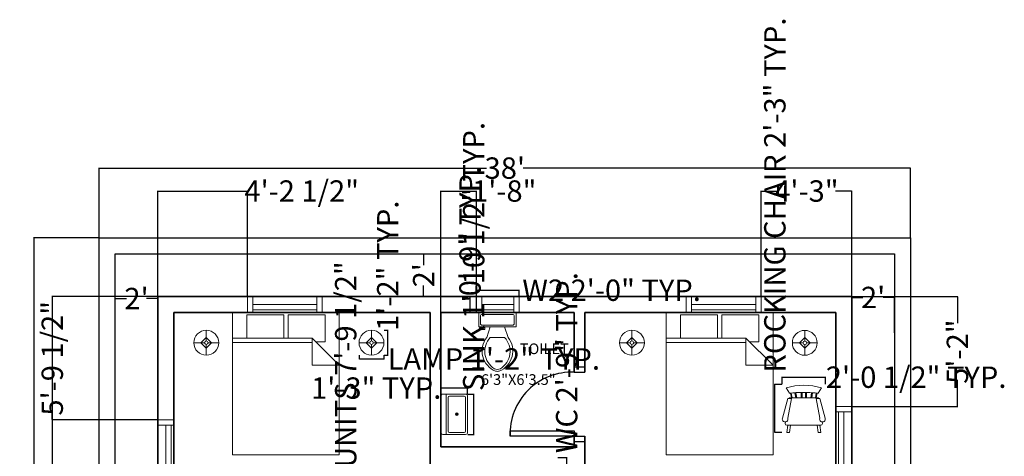
# Model space of a CAD drawing. Units: inches. Extents: x -107 to 531, y -526 to 131.
# Tile 4 of 4: x -23 to 531, y -114 to 131. Entities that reach past the tile are written whole.
import ezdxf

# ---------------------------------------------------------------- set-up
doc = ezdxf.new("R2010")
doc.units = ezdxf.units.IN
doc.header["$MEASUREMENT"] = 0
for name, color, linetype, lineweight in [('A-ANNO-DIMS', 2, 'Continuous', 18), ('A-AREA-IDEN', 7, 'Continuous', 25), ('A-DOOR', 3, 'Continuous', 25), ('A-FLOR-FIXT', 9, 'Continuous', 18), ('A-FURN', 8, 'Continuous', 18), ('A-GLAZ', 4, 'Continuous', 18), ('A-WALL', 7, 'Continuous', 35), ('C-PROP', 8, 'Continuous', 25)]:
    doc.layers.add(name, color=color, linetype=linetype, lineweight=lineweight)
doc.styles.get("Standard").update_dxf_attribs({"font": 'arial.ttf'})
doc.dimstyles.get("Standard").update_dxf_attribs({"dimtxt": 12, "dimasz": 0.18, "dimexe": 0.18, "dimexo": 0.0625, "dimgap": 0.09, "dimtad": 0, "dimdec": 1, "dimzin": 0, "dimdsep": 46, "dimlunit": 3, "dimtxsty": 'Standard', "dimcen": 0.09, "dimadec": 0, "dimazin": 0, "dimtfac": 1, "dimtdec": 1, "dimtofl": 0, "dimtmove": 0, "dimatfit": 3, "dimfxl": 1, "dimtolj": 1, "dimtzin": 0, "dimarcsym": 0})

# ---------------------------------------------------------------- blocks, each defined once
blk = doc.blocks.new('*D1')
at = {"layer": 'A-ANNO-DIMS', "color": 0, "lineweight": -2, "transparency": 16777216}
for p, q in [((21.95, 8.7), (21.95, 48.06)), ((22.13, 47.88), (239.68, 47.88)), ((477.77, 47.88), (260.22, 47.88)), ((477.95, 8.7), (477.95, 48.06))]:
    blk.add_line(p, q, dxfattribs=at)
at = {"layer": 'A-ANNO-DIMS', "color": 0, "transparency": 16777216}
for points in [[(22.13, 47.91), (22.13, 47.85), (21.95, 47.88)], [(477.77, 47.91), (477.77, 47.85), (477.95, 47.88)]]:
    blk.add_solid(points, dxfattribs=at)
at = {"layer": 'Defpoints', "color": 0, "transparency": 16777216}
for p in [(477.95, 47.88), (21.95, 8.64), (477.95, 8.64)]:
    blk.add_point(p, dxfattribs=at)
at = {"layer": 'A-ANNO-DIMS', "color": 0, "transparency": 16777216, "insert": (249.95, 47.88), "char_height": 12, "attachment_point": 5}
blk.add_mtext("\\A1;38'", dxfattribs=at)
blk = doc.blocks.new('Bed - Queen')
for p, q in [((0, -80.00003), (0, 0)), ((0, 0), (59.99999, 0)), ((59.99999, 0), (59.99999, -80.00003)), ((7.99999, -1.2), (28.79998, -1.2)), ((7.99999, -14.4), (7.99999, -1.2)), ((28.79998, -1.2), (28.79998, -14.4)), ((31.19999, -1.2), (51.99999, -1.2)), ((31.19999, -14.4), (31.19999, -1.2)), ((51.99999, -1.2), (51.99999, -16.4)), ((0, -14.4), (44.8, -14.4)), ((59.99999, -29.6), (44.8, -14.4)), ((44.8, -14.4), (44.8, -29.6)), ((51.99999, -16.4), (46.79936, -16.4)), ((44.8, -16.8), (0, -16.8)), ((44.8, -29.6), (59.99999, -29.6)), ((59.99999, -80.00003), (0, -80.00003))]:
    blk.add_line(p, q)
blk = doc.blocks.new('Lamp - Table')
for p, q in [((0, 7), (0, 1)), ((-1, 0), (-7, 0)), ((0, 3), (-3, 0)), ((-3, 0), (0, -3)), ((3, 0), (0, 3)), ((0, -3), (3, 0)), ((1, 0), (7, 0)), ((0, -1), (0, -7))]:
    blk.add_line(p, q)
for radius in [7, 1]:
    blk.add_circle((0, 0), radius)
blk = doc.blocks.new('Toilet - top')
for p, q in [((9.5, -6), (9.5, -2)), ((-10, -8.5), (-8, -8.5)), ((-10, -9.5), (-10, -8.5)), ((-7, -9.5), (-10, -9.5)), ((-8, -8.5), (-8, -8)), ((-7, -8), (-7, -9.5)), ((-4, -8), (-6, -14)), ((4, -8), (6, -14)), ((4, -14), (-4, -14))]:
    blk.add_line(p, q)
blk.add_lwpolyline([(10.5, -8), (10.5, 0), (-10.5, 0), (-10.5, -8)], close=True)
for points in [[(-9.5, -2), (-9.5, -6)], [(8.5, -1), (-8.5, -1)], [(-8.5, -7), (8.5, -7)]]:
    blk.add_lwpolyline(points)
for centre, radius, start, end in [((-8.62, -1.88), 0.884, 81.8699, 188.1301), ((8.62, -1.88), 0.884, 351.8699, 98.1301), ((-8.62, -6.12), 0.884, 171.8699, 278.1301), ((8.62, -6.12), 0.884, 261.8699, 8.1301), ((3.52, -21.58), 12.17, 141.4691, 247.9714), ((4.2, -21.82), 11.33, 136.3677, 238.9468), ((-3.52, -21.58), 12.17, 292.0284, 38.5307), ((-4.2, -21.82), 11.33, 301.053, 43.6321), ((0, -27.88), 4, 245.7318, 294.2682), ((0, -29), 4, 254.8605, 285.1395)]:
    blk.add_arc(centre, radius, start, end)
blk = doc.blocks.new('Sink-single - 30 in top')
blk.add_line((-15, -3.999996), (15, -3.999996))
for points in [[(-13.5, 0), (13.5, 0)], [(-15, -18.499996), (-15, -1.5)], [(-13.5, -17.499996), (-13.5, -6.499996)], [(-12.5, -5.499996), (12.5, -5.499996)], [(13.5, -6.499996), (13.5, -17.499996)], [(15, -1.5), (15, -18.499996)], [(13.5, -19.999996), (-13.5, -19.999996)], [(12.5, -18.499996), (-12.5, -18.499996)]]:
    blk.add_lwpolyline(points)
for radius in [1, 0.5]:
    blk.add_circle((0, -11.999996), radius)
for centre, radius, start, end in [((-13.5, -1.5), 1.5, 90, 180), ((-12.5, -6.499996), 1, 90, 180), ((12.5, -6.499996), 1, 0, 90), ((13.5, -1.5), 1.5, 0, 90), ((-13.5, -18.499996), 1.5, 180, 270), ((-12.5, -17.499996), 1, 180, 270), ((12.5, -17.499996), 1, 270, 0), ((13.5, -18.499996), 1.5, 270, 0)]:
    blk.add_arc(centre, radius, start, end)
blk = doc.blocks.new('*D13')
at = {"layer": 'A-ANNO-DIMS', "color": 0, "lineweight": -2, "transparency": 16777216}
for p, q in [((444.95, -44.8), (444.95, -24.66)), ((445.13, -24.84), (451.24, -24.84)), ((468.77, -24.84), (462.66, -24.84)), ((468.95, -44.8), (468.95, -24.66))]:
    blk.add_line(p, q, dxfattribs=at)
at = {"layer": 'A-ANNO-DIMS', "color": 0, "transparency": 16777216}
for points in [[(445.13, -24.81), (445.13, -24.87), (444.95, -24.84)], [(468.77, -24.81), (468.77, -24.87), (468.95, -24.84)]]:
    blk.add_solid(points, dxfattribs=at)
at = {"layer": 'Defpoints', "color": 0, "transparency": 16777216}
for p in [(468.95, -24.84), (444.95, -44.86), (468.95, -44.86)]:
    blk.add_point(p, dxfattribs=at)
at = {"layer": 'A-ANNO-DIMS', "color": 0, "transparency": 16777216, "insert": (456.95, -24.84), "char_height": 12, "attachment_point": 5}
blk.add_mtext("\\A1;2'", dxfattribs=at)
blk = doc.blocks.new('*D14')
at = {"layer": 'A-ANNO-DIMS', "color": 0, "lineweight": -2, "transparency": 16777216}
for p, q in [((30.95, -34.2), (30.95, -25.25)), ((31.13, -25.43), (37.24, -25.43)), ((54.77, -25.43), (48.66, -25.43)), ((54.95, -34.2), (54.95, -25.25))]:
    blk.add_line(p, q, dxfattribs=at)
at = {"layer": 'A-ANNO-DIMS', "color": 0, "transparency": 16777216}
for points in [[(31.13, -25.4), (31.13, -25.46), (30.95, -25.43)], [(54.77, -25.4), (54.77, -25.46), (54.95, -25.43)]]:
    blk.add_solid(points, dxfattribs=at)
at = {"layer": 'Defpoints', "color": 0, "transparency": 16777216}
for p in [(30.95, -25.43), (30.95, -34.26), (54.95, -34.26)]:
    blk.add_point(p, dxfattribs=at)
at = {"layer": 'A-ANNO-DIMS', "color": 0, "transparency": 16777216, "insert": (42.95, -25.43), "char_height": 12, "attachment_point": 5}
blk.add_mtext("\\A1;2'", dxfattribs=at)
blk = doc.blocks.new('*D15')
at = {"layer": 'A-ANNO-DIMS', "color": 0, "lineweight": -2, "transparency": 16777216}
for p, q in [((196.15, -0.36), (204.52, -0.36)), ((204.34, -0.54), (204.34, -6.65)), ((204.34, -24.18), (204.34, -18.08)), ((196.15, -24.36), (204.52, -24.36))]:
    blk.add_line(p, q, dxfattribs=at)
at = {"layer": 'A-ANNO-DIMS', "color": 0, "transparency": 16777216}
for points in [[(204.31, -0.54), (204.37, -0.54), (204.34, -0.36)], [(204.31, -24.18), (204.37, -24.18), (204.34, -24.36)]]:
    blk.add_solid(points, dxfattribs=at)
at = {"layer": 'Defpoints', "color": 0, "transparency": 16777216}
for p in [(196.09, -0.36), (204.34, -0.36), (196.09, -24.36)]:
    blk.add_point(p, dxfattribs=at)
at = {"layer": 'A-ANNO-DIMS', "color": 0, "transparency": 16777216, "insert": (204.34, -12.36), "char_height": 12, "attachment_point": 5, "rotation": 90}
blk.add_mtext("\\A1;2'", dxfattribs=at)
blk = doc.blocks.new('Chair - Rocking')
for p, q in [((-8, -4.5), (-10, -1.5)), ((-7.5, -4.5), (-7, -7)), ((-6.5, -7), (-7.02225, -4.43)), ((-4.5, -7), (-4.96674, -4.19951)), ((-4, -7), (-4.40532, -4.16272)), ((-1.5, -4.05012), (-1.5, -7)), ((-1, -7), (-1, -4.05012)), ((1, -7), (1, -4.04655)), ((1.5, -4.05012), (1.5, -7)), ((4, -7), (4.40187, -4.18694)), ((4.5, -7), (4.96761, -4.19437)), ((6.5, -7), (7, -4.4057)), ((7.5, -4.5), (7, -7)), ((8, -4.5), (10, -1.5)), ((-9, -7.5), (-12, -18.49999)), ((-7, -7.5), (-9, -7.5)), ((-9, -18.49999), (-7, -7.5)), ((-8.23428, -6.99939), (-8.3093, -7.47958)), ((-8.23041, -7), (8.23915, -7)), ((7, -7.5), (9, -7.5)), ((9, -18.49999), (7, -7.5)), ((8.31071, -7.48854), (8.23449, -7.00073)), ((9, -7.5), (12, -18.49999)), ((-10.36644, -20.64523), (-10.5, -21.49999)), ((10.5, -21.49999), (10.3575, -20.58798)), ((-9, -22.49999), (-9.5, -26.49999)), ((0, -22.49999), (-9.5, -22.49999)), ((-9.5, -26.49999), (-8, -26.49999)), ((-8, -26.49999), (-7.5, -22.49999)), ((0, -22.49999), (9.5, -22.49999)), ((8, -26.49999), (7.5, -22.49999)), ((9.5, -26.49999), (8, -26.49999)), ((9, -22.49999), (9.5, -26.49999))]:
    blk.add_line(p, q)
for centre, radius, start, end in [((0, -34.08333), 34.08333, 72.93847, 107.0615), ((0, -68.25004), 64.25, 93.92211, 97.15267), ((0, -68.25004), 64.25, 82.84733, 93.92211), ((-10.5, -18.99999), 1.58114, 161.5651, 18.43495), ((-9.5, -21.49999), 1, 180, 270), ((10.5, -18.99999), 1.58114, 161.5651, 18.43495), ((9.5, -21.49999), 1, 270, 0)]:
    blk.add_arc(centre, radius, start, end)
blk = doc.blocks.new('*D18')
at = {"layer": 'A-ANNO-DIMS', "color": 0, "lineweight": -2, "transparency": 16777216}
for p, q in [((21.89, 8.64), (-15.01, 8.64)), ((-14.83, 8.46), (-14.83, -220.85)), ((-14.83, -471.18), (-14.83, -241.88)), ((21.89, -471.36), (-15.01, -471.36))]:
    blk.add_line(p, q, dxfattribs=at)
at = {"layer": 'A-ANNO-DIMS', "color": 0, "transparency": 16777216}
for points in [[(-14.86, 8.46), (-14.8, 8.46), (-14.83, 8.64)], [(-14.86, -471.18), (-14.8, -471.18), (-14.83, -471.36)]]:
    blk.add_solid(points, dxfattribs=at)
at = {"layer": 'Defpoints', "color": 0, "transparency": 16777216}
for p in [(21.95, 8.64), (-14.83, -471.36), (21.95, -471.36)]:
    blk.add_point(p, dxfattribs=at)
at = {"layer": 'A-ANNO-DIMS', "color": 0, "transparency": 16777216, "insert": (-14.83, -231.36), "char_height": 12, "attachment_point": 5, "rotation": 90}
blk.add_mtext("\\A1;40'", dxfattribs=at)
blk = doc.blocks.new('WIN-36')
for p, q in [((0, 0), (0, 9)), ((3, 0), (3, 9)), ((3, 9), (39, 9)), ((39, 7.5), (3, 7.5)), ((39, 9), (39, 0)), ((42, 9), (42, 0)), ((39, 4.5), (3, 4.5)), ((39, 0), (3, 0))]:
    blk.add_line(p, q)
blk = doc.blocks.new('WIN-18')
for p, q in [((0, 9), (0, 0)), ((21, 9), (3, 9)), ((3, 9), (3, 0)), ((21, 0), (21, 9)), ((24, 0), (24, 9)), ((3, 4.5), (21, 4.5)), ((3, 1.5), (21, 1.5)), ((3, 0), (21, 0))]:
    blk.add_line(p, q)
blk = doc.blocks.new('DOOR-36-SWING')
for p, q in [((36.03, 42), (42.03, 42)), ((36.03, 39), (42.03, 39)), ((36.03, 3), (42.03, 3)), ((36.03, 0), (42.03, 0))]:
    blk.add_line(p, q)
blk.add_lwpolyline([(36.03, 3), (0.03, 3), (0.03, 6), (36.03, 6)], close=True)
blk.add_arc((34.53, 4.5), 34.53, 87.5104, 182.4896)
blk = doc.blocks.new('*D25')
at = {"layer": 'A-ANNO-DIMS', "color": 0, "lineweight": -2, "transparency": 16777216}
for p, q in [((233.99, -24.3), (233.99, -20.58)), ((234.17, -20.76), (257.81, -20.76)), ((257.99, -24.3), (257.99, -20.58)), ((257.99, -20.76), (258.17, -20.76))]:
    blk.add_line(p, q, dxfattribs=at)
at = {"layer": 'A-ANNO-DIMS', "color": 0, "transparency": 16777216}
for points in [[(234.17, -20.73), (234.17, -20.79), (233.99, -20.76)], [(257.81, -20.73), (257.81, -20.79), (257.99, -20.76)]]:
    blk.add_solid(points, dxfattribs=at)
at = {"layer": 'Defpoints', "color": 0, "transparency": 16777216}
for p in [(257.99, -20.76), (233.99, -24.36), (257.99, -24.36)]:
    blk.add_point(p, dxfattribs=at)
at = {"layer": 'A-ANNO-DIMS', "color": 0, "transparency": 16777216, "insert": (309.98, -20.76), "char_height": 12, "attachment_point": 5}
blk.add_mtext('\\A1;W2 2\'-0" TYP.', dxfattribs=at)
blk = doc.blocks.new('*D26')
at = {"layer": 'A-ANNO-DIMS', "color": 0, "lineweight": -2, "transparency": 16777216}
for p, q in [((233.93, -24.36), (230.21, -24.36)), ((230.39, -24.36), (230.39, -24.18)), ((230.39, -33.18), (230.39, -24.54)), ((233.93, -33.36), (230.21, -33.36))]:
    blk.add_line(p, q, dxfattribs=at)
at = {"layer": 'A-ANNO-DIMS', "color": 0, "transparency": 16777216}
for points in [[(230.36, -24.54), (230.42, -24.54), (230.39, -24.36)], [(230.36, -33.18), (230.42, -33.18), (230.39, -33.36)]]:
    blk.add_solid(points, dxfattribs=at)
at = {"layer": 'Defpoints', "color": 0, "transparency": 16777216}
for p in [(230.39, -24.36), (233.99, -24.36), (233.99, -33.36)]:
    blk.add_point(p, dxfattribs=at)
at = {"layer": 'A-ANNO-DIMS', "color": 0, "transparency": 16777216, "insert": (230.39, 12.48), "char_height": 12, "attachment_point": 5, "rotation": 90}
blk.add_mtext('\\A1;0\'-9" TYP.', dxfattribs=at)
blk = doc.blocks.new('*D33')
at = {"layer": 'A-ANNO-DIMS', "color": 0, "lineweight": -2, "transparency": 16777216}
for p, q in [((168.03, -57.34), (168.03, -59.56)), ((168.21, -59.38), (181.85, -59.38)), ((182.03, -57.34), (182.03, -59.56)), ((182.03, -59.38), (182.21, -59.38))]:
    blk.add_line(p, q, dxfattribs=at)
at = {"layer": 'A-ANNO-DIMS', "color": 0, "transparency": 16777216}
for points in [[(168.21, -59.35), (168.21, -59.41), (168.03, -59.38)], [(181.85, -59.35), (181.85, -59.41), (182.03, -59.38)]]:
    blk.add_solid(points, dxfattribs=at)
at = {"layer": 'Defpoints', "color": 0, "transparency": 16777216}
for p in [(168.03, -57.28), (182.03, -57.28), (182.03, -59.38)]:
    blk.add_point(p, dxfattribs=at)
at = {"layer": 'A-ANNO-DIMS', "color": 0, "transparency": 16777216, "insert": (243.76, -59.38), "char_height": 12, "attachment_point": 5}
blk.add_mtext('\\A1;LAMP 1\'-2" TYP.', dxfattribs=at)
blk = doc.blocks.new('*D34')
at = {"layer": 'A-ANNO-DIMS', "color": 0, "lineweight": -2, "transparency": 16777216}
for p, q in [((182.09, -43.28), (184.31, -43.28)), ((184.13, -43.28), (184.13, -43.1)), ((184.13, -57.1), (184.13, -43.46)), ((182.09, -57.28), (184.31, -57.28))]:
    blk.add_line(p, q, dxfattribs=at)
at = {"layer": 'A-ANNO-DIMS', "color": 0, "transparency": 16777216}
for points in [[(184.1, -43.46), (184.16, -43.46), (184.13, -43.28)], [(184.1, -57.1), (184.16, -57.1), (184.13, -57.28)]]:
    blk.add_solid(points, dxfattribs=at)
at = {"layer": 'Defpoints', "color": 0, "transparency": 16777216}
for p in [(182.03, -43.28), (184.13, -43.28), (182.03, -57.28)]:
    blk.add_point(p, dxfattribs=at)
at = {"layer": 'A-ANNO-DIMS', "color": 0, "transparency": 16777216, "insert": (184.13, -7), "char_height": 12, "attachment_point": 5, "rotation": 90}
blk.add_mtext('\\A1;1\'-2" TYP.', dxfattribs=at)
blk = doc.blocks.new('*D35')
at = {"layer": 'A-ANNO-DIMS', "color": 0, "lineweight": -2, "transparency": 16777216}
for p, q in [((405.71, -73.69), (401.54, -73.69)), ((401.72, -73.69), (401.72, -73.51)), ((401.72, -100.51), (401.72, -73.87)), ((405.71, -100.69), (401.54, -100.69))]:
    blk.add_line(p, q, dxfattribs=at)
at = {"layer": 'A-ANNO-DIMS', "color": 0, "transparency": 16777216}
for points in [[(401.69, -73.87), (401.75, -73.87), (401.72, -73.69)], [(401.69, -100.51), (401.75, -100.51), (401.72, -100.69)]]:
    blk.add_solid(points, dxfattribs=at)
at = {"layer": 'Defpoints', "color": 0, "transparency": 16777216}
for p in [(401.72, -73.69), (405.77, -73.69), (405.77, -100.69)]:
    blk.add_point(p, dxfattribs=at)
at = {"layer": 'A-ANNO-DIMS', "color": 0, "transparency": 16777216, "insert": (401.72, 32.7), "char_height": 12, "attachment_point": 5, "rotation": 90}
blk.add_mtext('\\A1;ROCKING CHAIR 2\'-3" TYP.', dxfattribs=at)
blk = doc.blocks.new('*D36')
at = {"layer": 'A-ANNO-DIMS', "color": 0, "lineweight": -2, "transparency": 16777216}
for p, q in [((405.77, -73.63), (405.77, -69.46)), ((405.95, -69.64), (430.02, -69.64)), ((430.2, -73.63), (430.2, -69.46)), ((430.2, -69.64), (430.38, -69.64))]:
    blk.add_line(p, q, dxfattribs=at)
at = {"layer": 'A-ANNO-DIMS', "color": 0, "transparency": 16777216}
for points in [[(405.95, -69.61), (405.95, -69.67), (405.77, -69.64)], [(430.02, -69.61), (430.02, -69.67), (430.2, -69.64)]]:
    blk.add_solid(points, dxfattribs=at)
at = {"layer": 'Defpoints', "color": 0, "transparency": 16777216}
for p in [(430.2, -69.64), (405.77, -73.69), (430.2, -73.69)]:
    blk.add_point(p, dxfattribs=at)
at = {"layer": 'A-ANNO-DIMS', "color": 0, "transparency": 16777216, "insert": (481.13, -69.64), "char_height": 12, "attachment_point": 5}
blk.add_mtext('\\A1;2\'-0 1/2" TYP.', dxfattribs=at)
blk = doc.blocks.new('*D39')
at = {"layer": 'A-ANNO-DIMS', "color": 0, "lineweight": -2, "transparency": 16777216}
for p, q in [((229.12, -79.16), (232.64, -79.16)), ((232.46, -79.16), (232.46, -78.98)), ((232.46, -101.64), (232.46, -79.34)), ((229.12, -101.82), (232.64, -101.82))]:
    blk.add_line(p, q, dxfattribs=at)
at = {"layer": 'A-ANNO-DIMS', "color": 0, "transparency": 16777216}
for points in [[(232.43, -79.34), (232.49, -79.34), (232.46, -79.16)], [(232.43, -101.64), (232.49, -101.64), (232.46, -101.82)]]:
    blk.add_solid(points, dxfattribs=at)
at = {"layer": 'Defpoints', "color": 0, "transparency": 16777216}
for p in [(229.06, -79.16), (232.46, -79.16), (229.06, -101.82)]:
    blk.add_point(p, dxfattribs=at)
at = {"layer": 'A-ANNO-DIMS', "color": 0, "transparency": 16777216, "insert": (232.46, -1.81), "char_height": 12, "attachment_point": 5, "rotation": 90}
blk.add_mtext('\\A1;SINK 1\'-10 1/2" TYP.', dxfattribs=at)
blk = doc.blocks.new('*D40')
at = {"layer": 'A-ANNO-DIMS', "color": 0, "lineweight": -2, "transparency": 16777216}
for p, q in [((213.95, -75.76), (213.77, -75.76)), ((213.95, -79.09), (213.95, -75.58)), ((228.88, -75.76), (214.13, -75.76)), ((229.06, -79.09), (229.06, -75.58))]:
    blk.add_line(p, q, dxfattribs=at)
at = {"layer": 'A-ANNO-DIMS', "color": 0, "transparency": 16777216}
for points in [[(214.13, -75.73), (214.13, -75.79), (213.95, -75.76)], [(228.88, -75.73), (228.88, -75.79), (229.06, -75.76)]]:
    blk.add_solid(points, dxfattribs=at)
at = {"layer": 'Defpoints', "color": 0, "transparency": 16777216}
for p in [(213.95, -75.76), (213.95, -79.16), (229.06, -79.16)]:
    blk.add_point(p, dxfattribs=at)
at = {"layer": 'A-ANNO-DIMS', "color": 0, "transparency": 16777216, "insert": (177.67, -75.76), "char_height": 12, "attachment_point": 5}
blk.add_mtext('\\A1;1\'-3" TYP.', dxfattribs=at)
blk = doc.blocks.new('*D43')
at = {"layer": 'A-ANNO-DIMS', "color": 0, "lineweight": -2, "transparency": 16777216}
for p, q in [((279.83, -114.86), (284.9, -114.86)), ((284.72, -114.86), (284.72, -114.68)), ((284.72, -147.73), (284.72, -115.04)), ((279.83, -147.91), (284.9, -147.91))]:
    blk.add_line(p, q, dxfattribs=at)
at = {"layer": 'A-ANNO-DIMS', "color": 0, "transparency": 16777216}
for points in [[(284.69, -115.04), (284.75, -115.04), (284.72, -114.86)], [(284.69, -147.73), (284.75, -147.73), (284.72, -147.91)]]:
    blk.add_solid(points, dxfattribs=at)
at = {"layer": 'Defpoints', "color": 0, "transparency": 16777216}
for p in [(279.77, -114.86), (284.72, -114.86), (279.77, -147.91)]:
    blk.add_point(p, dxfattribs=at)
at = {"layer": 'A-ANNO-DIMS', "color": 0, "transparency": 16777216, "insert": (284.72, -61.48), "char_height": 12, "attachment_point": 5, "rotation": 90}
blk.add_mtext('\\A1;WC 2\'-9" TYP.', dxfattribs=at)
blk = doc.blocks.new('*D51')
at = {"layer": 'A-ANNO-DIMS', "color": 0, "lineweight": -2, "transparency": 16777216}
for p, q in [((146.59, -195.42), (160.7, -195.42)), ((160.52, -195.42), (160.52, -195.24)), ((160.52, -288.52), (160.52, -195.6)), ((146.59, -288.7), (160.7, -288.7))]:
    blk.add_line(p, q, dxfattribs=at)
at = {"layer": 'A-ANNO-DIMS', "color": 0, "transparency": 16777216}
for points in [[(160.49, -195.6), (160.55, -195.6), (160.52, -195.42)], [(160.49, -288.52), (160.55, -288.52), (160.52, -288.7)]]:
    blk.add_solid(points, dxfattribs=at)
at = {"layer": 'Defpoints', "color": 0, "transparency": 16777216}
for p in [(146.53, -195.42), (160.52, -195.42), (146.53, -288.7)]:
    blk.add_point(p, dxfattribs=at)
at = {"layer": 'A-ANNO-DIMS', "color": 0, "transparency": 16777216, "insert": (160.52, -98.9), "char_height": 12, "attachment_point": 5, "rotation": 90}
blk.add_mtext('\\A1;KITCHEN UNITS 7\'-9 1/2"', dxfattribs=at)
blk = doc.blocks.new('*D60')
at = {"layer": 'A-ANNO-DIMS', "color": 0, "lineweight": -2, "transparency": 16777216}
for p, q in [((54.89, -24.36), (-4.58, -24.36)), ((-4.4, -24.54), (-4.4, -227.16)), ((-4.4, -471.18), (-4.4, -268.56)), ((21.89, -471.36), (-4.58, -471.36))]:
    blk.add_line(p, q, dxfattribs=at)
at = {"layer": 'A-ANNO-DIMS', "color": 0, "transparency": 16777216}
for points in [[(-4.43, -24.54), (-4.37, -24.54), (-4.4, -24.36)], [(-4.43, -471.18), (-4.37, -471.18), (-4.4, -471.36)]]:
    blk.add_solid(points, dxfattribs=at)
at = {"layer": 'Defpoints', "color": 0, "transparency": 16777216}
for p in [(54.95, -24.36), (-4.4, -471.36), (21.95, -471.36)]:
    blk.add_point(p, dxfattribs=at)
at = {"layer": 'A-ANNO-DIMS', "color": 0, "transparency": 16777216, "insert": (-4.4, -247.86), "char_height": 12, "attachment_point": 5, "rotation": 90}
blk.add_mtext('\\A1;37\'-3"', dxfattribs=at)
blk = doc.blocks.new('*D63')
at = {"layer": 'A-ANNO-DIMS', "color": 0, "lineweight": -2, "transparency": 16777216}
for p, q in [((54.95, -24.3), (54.95, 35.17)), ((55.13, 34.99), (105.17, 34.99)), ((105.35, -24.3), (105.35, 35.17)), ((105.35, 34.99), (105.53, 34.99))]:
    blk.add_line(p, q, dxfattribs=at)
at = {"layer": 'A-ANNO-DIMS', "color": 0, "transparency": 16777216}
for points in [[(55.13, 35.02), (55.13, 34.96), (54.95, 34.99)], [(105.17, 35.02), (105.17, 34.96), (105.35, 34.99)]]:
    blk.add_solid(points, dxfattribs=at)
at = {"layer": 'Defpoints', "color": 0, "transparency": 16777216}
for p in [(105.35, 34.99), (54.95, -24.36), (105.35, -24.36)]:
    blk.add_point(p, dxfattribs=at)
at = {"layer": 'A-ANNO-DIMS', "color": 0, "transparency": 16777216, "insert": (135.79, 34.99), "char_height": 12, "attachment_point": 5}
blk.add_mtext('\\A1;4\'-2 1/2"', dxfattribs=at)
blk = doc.blocks.new('*D64')
at = {"layer": 'A-ANNO-DIMS', "color": 0, "lineweight": -2, "transparency": 16777216}
for p, q in [((393.96, -24.3), (393.96, 35.17)), ((394.14, 34.99), (403.17, 34.99)), ((444.77, 34.99), (435.74, 34.99)), ((444.95, -24.3), (444.95, 35.17))]:
    blk.add_line(p, q, dxfattribs=at)
at = {"layer": 'A-ANNO-DIMS', "color": 0, "transparency": 16777216}
for points in [[(394.14, 35.02), (394.14, 34.96), (393.96, 34.99)], [(444.77, 35.02), (444.77, 34.96), (444.95, 34.99)]]:
    blk.add_solid(points, dxfattribs=at)
at = {"layer": 'Defpoints', "color": 0, "transparency": 16777216}
for p in [(444.95, 34.99), (393.96, -24.36), (444.95, -24.36)]:
    blk.add_point(p, dxfattribs=at)
at = {"layer": 'A-ANNO-DIMS', "color": 0, "transparency": 16777216, "insert": (419.46, 34.99), "char_height": 12, "attachment_point": 5}
blk.add_mtext('\\A1;4\'-3"', dxfattribs=at)
blk = doc.blocks.new('*D65')
at = {"layer": 'A-ANNO-DIMS', "color": 0, "lineweight": -2, "transparency": 16777216}
for p, q in [((213.95, -33.3), (213.95, 35.17)), ((214.13, 34.99), (233.81, 34.99)), ((233.99, -33.3), (233.99, 35.17)), ((233.99, 34.99), (234.17, 34.99))]:
    blk.add_line(p, q, dxfattribs=at)
at = {"layer": 'A-ANNO-DIMS', "color": 0, "transparency": 16777216}
for points in [[(214.13, 35.02), (214.13, 34.96), (213.95, 34.99)], [(233.81, 35.02), (233.81, 34.96), (233.99, 34.99)]]:
    blk.add_solid(points, dxfattribs=at)
at = {"layer": 'Defpoints', "color": 0, "transparency": 16777216}
for p in [(233.99, 34.99), (213.95, -33.36), (233.99, -33.36)]:
    blk.add_point(p, dxfattribs=at)
at = {"layer": 'A-ANNO-DIMS', "color": 0, "transparency": 16777216, "insert": (249.64, 34.99), "char_height": 12, "attachment_point": 5}
blk.add_mtext('\\A1;1\'-8"', dxfattribs=at)
blk = doc.blocks.new('*D70')
at = {"layer": 'A-ANNO-DIMS', "color": 0, "lineweight": -2, "transparency": 16777216}
for p, q in [((54.89, -24.36), (-4.58, -24.36)), ((-4.4, -24.54), (-4.4, -29)), ((54.89, -93.68), (-4.58, -93.68)), ((-4.4, -93.5), (-4.4, -89.04))]:
    blk.add_line(p, q, dxfattribs=at)
at = {"layer": 'A-ANNO-DIMS', "color": 0, "transparency": 16777216}
for points in [[(-4.43, -24.54), (-4.37, -24.54), (-4.4, -24.36)], [(-4.43, -93.5), (-4.37, -93.5), (-4.4, -93.68)]]:
    blk.add_solid(points, dxfattribs=at)
at = {"layer": 'Defpoints', "color": 0, "transparency": 16777216}
for p in [(54.95, -24.36), (-4.4, -93.68), (54.95, -93.68)]:
    blk.add_point(p, dxfattribs=at)
at = {"layer": 'A-ANNO-DIMS', "color": 0, "transparency": 16777216, "insert": (-4.4, -59.02), "char_height": 12, "attachment_point": 5, "rotation": 90}
blk.add_mtext('\\A1;5\'-9 1/2"', dxfattribs=at)
blk = doc.blocks.new('*D73')
at = {"layer": 'A-ANNO-DIMS', "color": 0, "lineweight": -2, "transparency": 16777216}
for p, q in [((445.01, -24.36), (504.48, -24.36)), ((504.3, -24.54), (504.3, -39.23)), ((504.3, -85.99), (504.3, -71.3)), ((445.01, -86.17), (504.48, -86.17))]:
    blk.add_line(p, q, dxfattribs=at)
at = {"layer": 'A-ANNO-DIMS', "color": 0, "transparency": 16777216}
for points in [[(504.27, -24.54), (504.33, -24.54), (504.3, -24.36)], [(504.27, -85.99), (504.33, -85.99), (504.3, -86.17)]]:
    blk.add_solid(points, dxfattribs=at)
at = {"layer": 'Defpoints', "color": 0, "transparency": 16777216}
for p in [(444.95, -24.36), (444.95, -86.17), (504.3, -86.17)]:
    blk.add_point(p, dxfattribs=at)
at = {"layer": 'A-ANNO-DIMS', "color": 0, "transparency": 16777216, "insert": (504.3, -55.27), "char_height": 12, "attachment_point": 5, "rotation": 90}
blk.add_mtext('\\A1;5\'-2"', dxfattribs=at)

msp = doc.modelspace()

# ---------------------------------------------------------------- linework, layer by layer
at = {"layer": 'A-WALL'}
for p, q in [((54.95, -462.36), (54.95, -24.36)), ((54.95, -24.36), (444.95, -24.36)), ((444.95, -24.36), (444.95, -462.36)), ((63.95, -33.36), (207.95, -33.36)), ((63.95, -189.36), (63.95, -33.36)), ((207.95, -120.86), (207.95, -33.36)), ((213.95, -108.86), (213.95, -33.36)), ((213.95, -33.36), (288.95, -33.36)), ((288.95, -66.86), (288.95, -33.36)), ((294.95, -66.86), (294.95, -33.36)), ((294.95, -33.36), (435.95, -33.36)), ((435.95, -33.36), (435.95, -189.36)), ((288.95, -108.86), (288.95, -102.86)), ((294.95, -189.36), (294.95, -102.86)), ((213.95, -108.86), (288.95, -108.86))]:
    msp.add_line(p, q, dxfattribs=at)
at = {"layer": 'C-PROP'}
for p, q in [((30.95, -0.36), (468.95, -0.36)), ((30.95, -462.36), (30.95, -0.36)), ((468.95, -0.36), (468.95, -462.36))]:
    msp.add_line(p, q, dxfattribs=at)
msp.add_lwpolyline([(231.95, -471.36), (21.95, -471.36), (21.95, 8.64), (477.95, 8.64), (477.95, -471.36), (303.95, -471.36)], dxfattribs=at)

# ---------------------------------------------------------------- block references
at = {"layer": 'A-DOOR'}
msp.add_blockref('DOOR-36-SWING', (252.92, -105.86), dxfattribs=at)
at = {"layer": 'A-FLOR-FIXT'}
msp.add_blockref('Toilet - top', (245.8, -33.36), dxfattribs=at)
at = {"layer": 'A-FLOR-FIXT', "xscale": 0.7554348055935636, "yscale": 0.7554348055935636, "zscale": 0.7554348055935636, "rotation": 90}
msp.add_blockref('Sink-single - 30 in top', (213.95, -90.49), dxfattribs=at)
at = {"layer": 'A-FURN'}
for name, p in [('Bed - Queen', (96.92, -33.36)), ('Bed - Queen', (340.7, -33.36)), ('Lamp - Table', (82.18, -50.28)), ('Lamp - Table', (175.03, -50.28)), ('Lamp - Table', (321.39, -50.28)), ('Lamp - Table', (418.55, -50.34)), ('Chair - Rocking', (417.99, -74.19))]:
    msp.add_blockref(name, p, dxfattribs=at)
at = {"layer": 'A-GLAZ'}
for p, rotation in [((147.35, -24.36), 180), ((393.96, -24.36), 180), ((444.95, -128.17), 89.99999999999987), ((54.95, -93.68), 270.0000000000002)]:
    msp.add_blockref('WIN-36', p, dxfattribs=dict(at, rotation=rotation))
msp.add_blockref('WIN-18', (233.99, -33.36), dxfattribs=at)

# ---------------------------------------------------------------- texts
at = {"layer": 'A-AREA-IDEN'}
for s, p in [('TOILET', (258.36, -56.68)), ('6\'3"X6\'3.5"', (236.54, -73.97))]:
    msp.add_text(s, height=6, dxfattribs=at).set_placement(p)

# ---------------------------------------------------------------- dimensions: what is measured, and where the dimension line sits
at = {"layer": 'A-ANNO-DIMS'}
for base, p1, p2, angle, text, picture, middle in [((401.72, -73.69), (405.77, -100.69), (405.77, -73.69), 90, 'ROCKING CHAIR <> TYP.', '*D35', (401.72, 32.7)), ((232.46, -79.16), (229.06, -101.82), (229.06, -79.16), 90, 'SINK <> TYP.', '*D39', (232.46, -1.81)), ((230.39, -24.36), (233.99, -33.36), (233.99, -24.36), 90, '<> TYP.', '*D26', (230.39, 12.48)), ((184.13, -43.28), (182.03, -57.28), (182.03, -43.28), 90, '<> TYP.', '*D34', (184.13, -7)), ((160.52, -195.42), (146.53, -288.7), (146.53, -195.42), 90, 'KITCHEN UNITS <>', '*D51', (160.52, -98.9)), ((284.7239, -114.8618), (279.7669, -147.9081), (279.7669, -114.8618), 90, 'WC <> TYP.', '*D43', (284.7239, -61.48)), ((213.95, -75.76), (229.06, -79.16), (213.95, -79.16), 180, '<> TYP.', '*D40', (177.67, -75.76))]:
    dim = msp.add_linear_dim(base=base, p1=p1, p2=p2, angle=angle, text=text, dimstyle='Standard', override={"dimdec": 1, "dimlfac": 1, "dimrnd": 0, "dimzin": 1, "dimdsep": 46, "dimlunit": 4, "dimfrac": 2}, dxfattribs=at)
    dim.commit()
    dim.dimension.update_dxf_attribs({"geometry": picture, "text_midpoint": middle})
for base, p1, p2, override, picture, middle in [((477.95, 47.88), (21.95, 8.64), (477.95, 8.64), {"dimclrd": 0, "dimclre": 0, "dimclrt": 0}, '*D1', (249.95, 47.88)), ((105.35, 34.99), (54.95, -24.36), (105.35, -24.36), {"dimdec": 1, "dimlfac": 1, "dimrnd": 0, "dimzin": 1, "dimdsep": 46, "dimlunit": 4, "dimfrac": 2}, '*D63', (135.79, 34.99)), ((233.99, 34.99), (213.95, -33.36), (233.99, -33.36), {"dimdec": 1, "dimlfac": 1, "dimrnd": 0, "dimzin": 1, "dimdsep": 46, "dimlunit": 4, "dimfrac": 2}, '*D65', (249.64, 34.99)), ((444.95, 34.99), (393.96, -24.36), (444.95, -24.36), {"dimdec": 1, "dimlfac": 1, "dimrnd": 0, "dimzin": 1, "dimdsep": 46, "dimlunit": 4, "dimfrac": 2}, '*D64', (419.46, 34.99)), ((30.95, -25.43), (54.95, -34.26), (30.95, -34.26), {"dimclrd": 0, "dimclre": 0, "dimclrt": 0}, '*D14', (42.95, -25.43)), ((468.95, -24.84), (444.95, -44.86), (468.95, -44.86), {"dimclrd": 0, "dimclre": 0, "dimclrt": 0}, '*D13', (456.95, -24.84))]:
    dim = msp.add_linear_dim(base=base, p1=p1, p2=p2, dimstyle='Standard', override=override, dxfattribs=at)
    dim.commit()
    dim.dimension.update_dxf_attribs({"geometry": picture, "text_midpoint": middle})
for base, p1, p2, override, picture, middle in [((-14.83, -471.36), (21.95, 8.64), (21.95, -471.36), {"dimclrd": 0, "dimclre": 0, "dimclrt": 0}, '*D18', (-14.83, -231.36)), ((204.34, -0.36), (196.09, -24.36), (196.09, -0.36), {"dimclrd": 0, "dimclre": 0, "dimclrt": 0}, '*D15', (204.34, -12.36)), ((-4.4, -93.68), (54.95, -24.36), (54.95, -93.68), {"dimdec": 1, "dimlfac": 1, "dimrnd": 0, "dimzin": 1, "dimdsep": 46, "dimlunit": 4, "dimfrac": 2}, '*D70', (-4.4, -59.02)), ((-4.4, -471.36), (54.95, -24.36), (21.95, -471.36), {"dimdec": 1, "dimlfac": 1, "dimrnd": 0, "dimzin": 1, "dimdsep": 46, "dimlunit": 4, "dimfrac": 2}, '*D60', (-4.4, -247.86)), ((504.3, -86.17), (444.95, -24.36), (444.95, -86.17), {"dimdec": 1, "dimlfac": 1, "dimrnd": 0, "dimzin": 1, "dimdsep": 46, "dimlunit": 4, "dimfrac": 2}, '*D73', (504.3, -55.27))]:
    dim = msp.add_linear_dim(base=base, p1=p1, p2=p2, angle=90, dimstyle='Standard', override=override, dxfattribs=at)
    dim.commit()
    dim.dimension.update_dxf_attribs({"geometry": picture, "text_midpoint": middle})
for base, p1, p2, text, picture, middle in [((257.99, -20.76), (233.99, -24.36), (257.99, -24.36), 'W2 <> TYP.', '*D25', (309.98, -20.76)), ((182.03, -59.38), (168.03, -57.28), (182.03, -57.28), 'LAMP <> TYP.', '*D33', (243.76, -59.38)), ((430.2, -69.64), (405.77, -73.69), (430.2, -73.69), '<> TYP.', '*D36', (481.13, -69.64))]:
    dim = msp.add_linear_dim(base=base, p1=p1, p2=p2, text=text, dimstyle='Standard', override={"dimdec": 1, "dimlfac": 1, "dimrnd": 0, "dimzin": 1, "dimdsep": 46, "dimlunit": 4, "dimfrac": 2}, dxfattribs=at)
    dim.commit()
    dim.dimension.update_dxf_attribs({"geometry": picture, "text_midpoint": middle})

doc.saveas('drawing.dxf')
